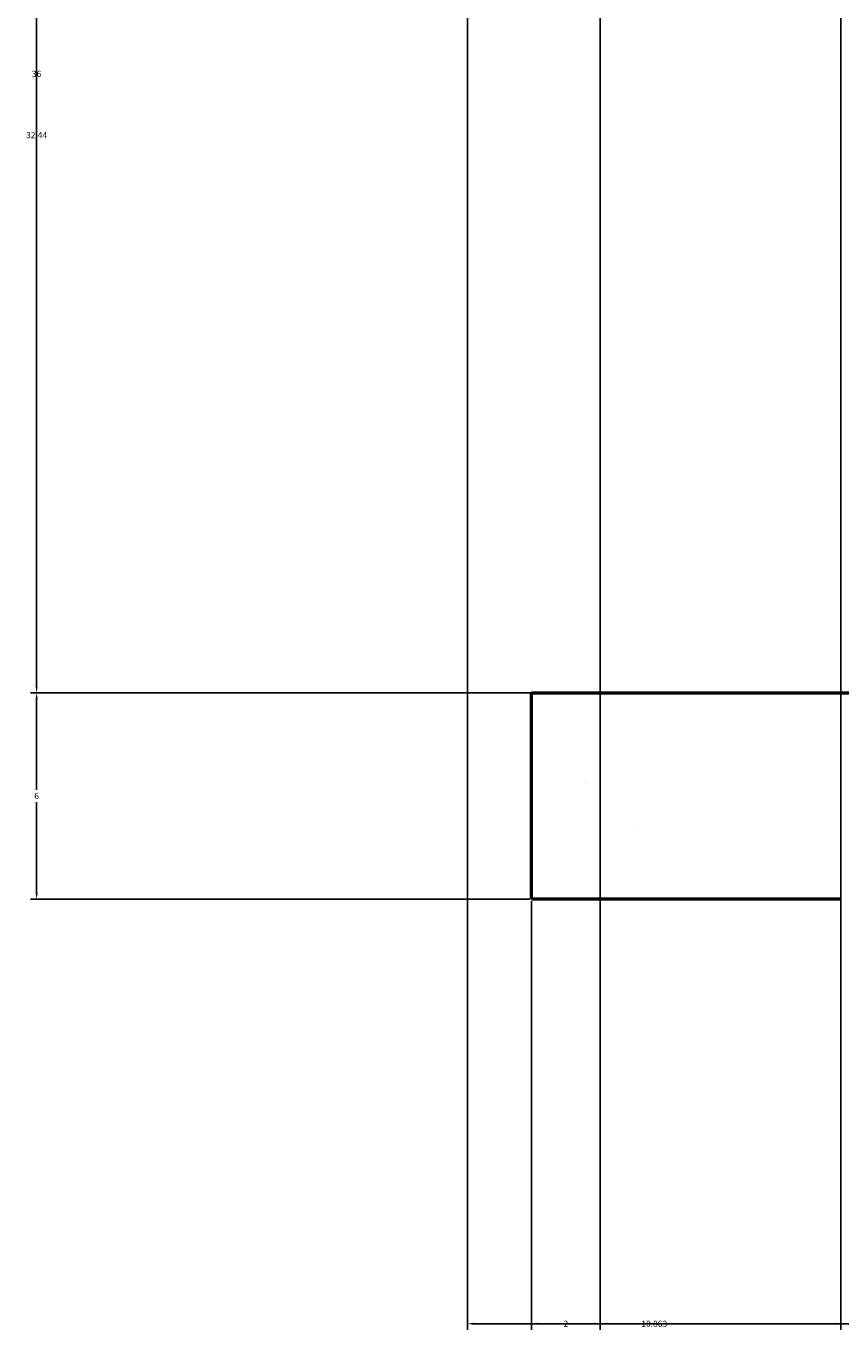
# Model space of a CAD drawing. Units: inches. Extents: x 2812 to 3051, y 1398 to 1659.
# Tile 1 of 65: x 2812 to 2835, y 1398 to 1435. Entities that reach past the tile are written whole.
import ezdxf

# ---------------------------------------------------------------- set-up
doc = ezdxf.new("R2010")
doc.units = ezdxf.units.IN
for name, color, linetype, lineweight in [('A-ANNO-DIMS', 2, 'Continuous', 18), ('S-CONC', 7, 'Continuous', 50), ('S-CONC-PATT', 8, 'Continuous', 18)]:
    doc.layers.add(name, color=color, linetype=linetype, lineweight=lineweight)
doc.styles.get("Standard").update_dxf_attribs({"font": 'arial.ttf'})
doc.dimstyles.get("Standard").update_dxf_attribs({"dimtxt": 0.18, "dimasz": 0.18, "dimexe": 0.18, "dimexo": 0.0625, "dimgap": 0.09, "dimtad": 0, "dimtih": 1, "dimtoh": 1, "dimdec": 4, "dimzin": 0, "dimdsep": 46, "dimtxsty": 'Standard', "dimcen": 0.09, "dimadec": 0, "dimazin": 0, "dimtfac": 1, "dimtdec": 4, "dimtofl": 0, "dimtmove": 0, "dimatfit": 3, "dimfxl": 1, "dimtolj": 1, "dimtzin": 0, "dimarcsym": 0})

# ---------------------------------------------------------------- blocks, each defined once
blk = doc.blocks.new('*D27')
at = {"layer": 'A-ANNO-DIMS', "color": 0, "lineweight": -2, "transparency": 16777216}
for p, q in [((2824.521, 1594.167), (2824.521, 1397.505)), ((2835.385, 1550.757), (2835.385, 1397.505)), ((2824.701, 1397.685), (2829.498, 1397.685)), ((2835.205, 1397.685), (2830.408, 1397.685))]:
    blk.add_line(p, q, dxfattribs=at)
at = {"layer": 'A-ANNO-DIMS', "color": 0, "transparency": 16777216}
for points in [[(2824.701, 1397.715), (2824.701, 1397.655), (2824.521, 1397.685)], [(2835.205, 1397.715), (2835.205, 1397.655), (2835.385, 1397.685)]]:
    blk.add_solid(points, dxfattribs=at)
at = {"layer": 'Defpoints', "color": 0, "transparency": 16777216}
for p in [(2824.521, 1594.23), (2835.385, 1550.82), (2835.385, 1397.685)]:
    blk.add_point(p, dxfattribs=at)
at = {"layer": 'A-ANNO-DIMS', "color": 0, "transparency": 16777216, "insert": (2829.953, 1397.685), "char_height": 0.18, "attachment_point": 5}
blk.add_mtext('\\A1;10.863', dxfattribs=at)
blk = doc.blocks.new('*D41')
at = {"layer": 'A-ANNO-DIMS', "color": 0, "lineweight": -2, "transparency": 16777216}
for p, q in [((2828.385, 1489.973), (2828.385, 1397.505)), ((2826.385, 1409.973), (2826.385, 1397.505)), ((2826.565, 1397.685), (2827.235, 1397.685)), ((2828.205, 1397.685), (2827.535, 1397.685))]:
    blk.add_line(p, q, dxfattribs=at)
at = {"layer": 'A-ANNO-DIMS', "color": 0, "transparency": 16777216}
for points in [[(2826.565, 1397.715), (2826.565, 1397.655), (2826.385, 1397.685)], [(2828.205, 1397.715), (2828.205, 1397.655), (2828.385, 1397.685)]]:
    blk.add_solid(points, dxfattribs=at)
at = {"layer": 'Defpoints', "color": 0, "transparency": 16777216}
for p in [(2828.385, 1490.035), (2826.385, 1410.035), (2828.385, 1397.685)]:
    blk.add_point(p, dxfattribs=at)
at = {"layer": 'A-ANNO-DIMS', "color": 0, "transparency": 16777216, "insert": (2827.385, 1397.685), "char_height": 0.18, "attachment_point": 5}
blk.add_mtext('\\A1;2', dxfattribs=at)
blk = doc.blocks.new('*D42')
at = {"layer": 'A-ANNO-DIMS', "color": 0, "lineweight": -2, "transparency": 16777216}
for p, q in [((2828.385, 1489.973), (2828.385, 1397.505)), ((2847.686, 1487.973), (2847.686, 1397.505)), ((2828.565, 1397.685), (2837.72, 1397.685)), ((2847.506, 1397.685), (2838.351, 1397.685))]:
    blk.add_line(p, q, dxfattribs=at)
at = {"layer": 'A-ANNO-DIMS', "color": 0, "transparency": 16777216}
for points in [[(2828.565, 1397.715), (2828.565, 1397.655), (2828.385, 1397.685)], [(2847.506, 1397.715), (2847.506, 1397.655), (2847.686, 1397.685)]]:
    blk.add_solid(points, dxfattribs=at)
at = {"layer": 'Defpoints', "color": 0, "transparency": 16777216}
for p in [(2828.385, 1490.035), (2847.686, 1488.035), (2847.686, 1397.685)]:
    blk.add_point(p, dxfattribs=at)
at = {"layer": 'A-ANNO-DIMS', "color": 0, "transparency": 16777216, "insert": (2838.036, 1397.685), "char_height": 0.18, "attachment_point": 5}
blk.add_mtext('\\A1;19.3', dxfattribs=at)
blk = doc.blocks.new('*D49')
at = {"layer": 'A-ANNO-DIMS', "color": 0, "lineweight": -2, "transparency": 16777216}
for p, q in [((2826.322, 1416.035), (2811.806, 1416.035)), ((2811.986, 1415.855), (2811.986, 1413.217)), ((2811.986, 1410.215), (2811.986, 1412.853)), ((2826.322, 1410.035), (2811.806, 1410.035))]:
    blk.add_line(p, q, dxfattribs=at)
at = {"layer": 'A-ANNO-DIMS', "color": 0, "transparency": 16777216}
for points in [[(2811.956, 1415.855), (2812.016, 1415.855), (2811.986, 1416.035)], [(2811.956, 1410.215), (2812.016, 1410.215), (2811.986, 1410.035)]]:
    blk.add_solid(points, dxfattribs=at)
at = {"layer": 'Defpoints', "color": 0, "transparency": 16777216}
for p in [(2811.986, 1416.035), (2826.385, 1416.035), (2826.385, 1410.035)]:
    blk.add_point(p, dxfattribs=at)
at = {"layer": 'A-ANNO-DIMS', "color": 0, "transparency": 16777216, "insert": (2811.986, 1413.035), "char_height": 0.18, "attachment_point": 5}
blk.add_mtext('\\A1;6', dxfattribs=at)
blk = doc.blocks.new('*D50')
at = {"layer": 'A-ANNO-DIMS', "color": 0, "lineweight": -2, "transparency": 16777216}
for p, q in [((2835.322, 1462.303), (2811.806, 1462.303)), ((2811.986, 1462.123), (2811.986, 1439.351)), ((2811.986, 1416.215), (2811.986, 1438.987)), ((2835.322, 1416.035), (2811.806, 1416.035))]:
    blk.add_line(p, q, dxfattribs=at)
at = {"layer": 'A-ANNO-DIMS', "color": 0, "transparency": 16777216}
for points in [[(2811.956, 1462.123), (2812.016, 1462.123), (2811.986, 1462.303)], [(2811.956, 1416.215), (2812.016, 1416.215), (2811.986, 1416.035)]]:
    blk.add_solid(points, dxfattribs=at)
at = {"layer": 'Defpoints', "color": 0, "transparency": 16777216}
for p in [(2811.986, 1462.303), (2835.385, 1462.303), (2835.385, 1416.035)]:
    blk.add_point(p, dxfattribs=at)
at = {"layer": 'A-ANNO-DIMS', "color": 0, "transparency": 16777216, "insert": (2811.986, 1439.169), "char_height": 0.18, "attachment_point": 5}
blk.add_mtext('\\A1;46.27', dxfattribs=at)
blk = doc.blocks.new('*D56')
at = {"layer": 'A-ANNO-DIMS', "color": 0, "lineweight": -2, "transparency": 16777216}
for p, q in [((2880.322, 1452.035), (2811.806, 1452.035)), ((2811.986, 1451.855), (2811.986, 1434.217)), ((2811.986, 1416.215), (2811.986, 1433.853)), ((2952.322, 1416.035), (2811.806, 1416.035))]:
    blk.add_line(p, q, dxfattribs=at)
at = {"layer": 'A-ANNO-DIMS', "color": 0, "transparency": 16777216}
for points in [[(2811.956, 1451.855), (2812.016, 1451.855), (2811.986, 1452.035)], [(2811.956, 1416.215), (2812.016, 1416.215), (2811.986, 1416.035)]]:
    blk.add_solid(points, dxfattribs=at)
at = {"layer": 'Defpoints', "color": 0, "transparency": 16777216}
for p in [(2811.986, 1452.035), (2880.385, 1452.035), (2952.385, 1416.035)]:
    blk.add_point(p, dxfattribs=at)
at = {"layer": 'A-ANNO-DIMS', "color": 0, "transparency": 16777216, "insert": (2811.986, 1434.035), "char_height": 0.18, "attachment_point": 5}
blk.add_mtext('\\A1;36', dxfattribs=at)
blk = doc.blocks.new('*D75')
at = {"layer": 'A-ANNO-DIMS', "color": 0, "lineweight": -2, "transparency": 16777216}
for p, q in [((2963.812, 1448.474), (2811.806, 1448.474)), ((2811.986, 1448.294), (2811.986, 1432.437)), ((2811.986, 1416.215), (2811.986, 1432.073)), ((2961.322, 1416.035), (2811.806, 1416.035))]:
    blk.add_line(p, q, dxfattribs=at)
at = {"layer": 'A-ANNO-DIMS', "color": 0, "transparency": 16777216}
for points in [[(2811.956, 1448.294), (2812.016, 1448.294), (2811.986, 1448.474)], [(2811.956, 1416.215), (2812.016, 1416.215), (2811.986, 1416.035)]]:
    blk.add_solid(points, dxfattribs=at)
at = {"layer": 'Defpoints', "color": 0, "transparency": 16777216}
for p in [(2811.986, 1448.474), (2963.874, 1448.474), (2961.385, 1416.035)]:
    blk.add_point(p, dxfattribs=at)
at = {"layer": 'A-ANNO-DIMS', "color": 0, "transparency": 16777216, "insert": (2811.986, 1432.255), "char_height": 0.18, "attachment_point": 5}
blk.add_mtext('\\A1;32.44', dxfattribs=at)

msp = doc.modelspace()

# ---------------------------------------------------------------- hatches: boundary and pattern name
at = {"layer": 'S-CONC-PATT'}
h = msp.add_hatch(dxfattribs=at)
h.set_pattern_fill('AR-SAND', color=256, scale=0.3)
h.paths.add_polyline_path([(3036.3849, 1416.0354), (3027.3849, 1416.0354), (2826.3849, 1416.0354), (2826.3849, 1410.0354), (2835.3849, 1410.0354), (3036.3849, 1410.0354)])
h.paths.add_polyline_path([(2970.3849, 1488.0354), (2969.3849, 1488.0354), (2941.3849, 1488.0354), (2941.3849, 1482.0354), (2970.3849, 1482.0354)])
h.paths.add_polyline_path([(3036.3849, 1488.0354), (3035.3849, 1488.0354), (3006.3849, 1488.0354), (3006.3849, 1482.0354), (3027.3849, 1482.0354), (3036.3849, 1482.0354)])
h.paths.add_polyline_path([(3034.3849, 1490.0354), (3008.3849, 1490.0354), (3008.3849, 1489.0354), (3034.3849, 1489.0354)])
h.paths.add_polyline_path([(3035.3849, 1489.0354), (3034.3849, 1489.0354), (3007.3849, 1489.0354), (3007.3849, 1488.0354), (3035.3849, 1488.0354)])
h.paths.add_polyline_path([(2968.3849, 1490.0354), (2943.3849, 1490.0354), (2943.3849, 1489.0354), (2968.3849, 1489.0354)])
h.paths.add_polyline_path([(2969.3849, 1489.0354), (2968.3849, 1489.0354), (2942.3849, 1489.0354), (2942.3849, 1488.0354), (2969.3849, 1488.0354)])
h.paths.add_polyline_path([(2896.3849, 1488.0354), (2826.3849, 1488.0354), (2826.3849, 1482.0354), (2896.3849, 1482.0354)])
h.paths.add_polyline_path([(2895.3849, 1489.0354), (2894.3849, 1489.0354), (2827.3849, 1489.0354), (2827.3849, 1488.0354), (2895.3849, 1488.0354)])
h.paths.add_polyline_path([(2894.3849, 1490.0354), (2828.3849, 1490.0354), (2828.3849, 1489.0354), (2894.3849, 1489.0354)])
h = msp.add_hatch(dxfattribs=at)
h.set_pattern_fill('AR-CONC', color=256, scale=0.3)
h.paths.add_polyline_path([(3036.3849, 1416.0354), (3027.3849, 1416.0354), (2826.3849, 1416.0354), (2826.3849, 1410.0354), (2835.3849, 1410.0354), (3036.3849, 1410.0354)])

# ---------------------------------------------------------------- linework, layer by layer
at = {"layer": 'S-CONC'}
for p, q in [((2826.3849, 1410.0354), (2826.3849, 1416.0354)), ((2826.3849, 1416.0354), (3027.3849, 1416.0354)), ((2835.3849, 1410.0354), (2826.3849, 1410.0354))]:
    msp.add_line(p, q, dxfattribs=at)

# ---------------------------------------------------------------- dimensions: what is measured, and where the dimension line sits
at = {"layer": 'A-ANNO-DIMS'}
for base, p1, p2, override, picture, middle in [((2835.384907, 1397.685398), (2824.521409, 1594.229631), (2835.384907, 1550.819971), {"dimdec": 3, "dimlfac": 1, "dimrnd": 0, "dimzin": 0, "dimdsep": 46, "dimlunit": 2}, '*D27', (2829.953158, 1397.685398)), ((2828.3849, 1397.6854), (2826.3849, 1410.0354), (2828.3849, 1490.0354), {"dimdec": 0, "dimlfac": 1, "dimrnd": 0, "dimzin": 0, "dimdsep": 46, "dimlunit": 2}, '*D41', (2827.3849, 1397.6854)), ((2847.6863, 1397.6854), (2828.3849, 1490.0354), (2847.6863, 1488.0354), {"dimdec": 1, "dimlfac": 1, "dimrnd": 0, "dimzin": 0, "dimdsep": 46, "dimlunit": 2}, '*D42', (2838.0356, 1397.6854))]:
    dim = msp.add_linear_dim(base=base, p1=p1, p2=p2, dimstyle='Standard', override=override, dxfattribs=at)
    dim.commit()
    dim.dimension.update_dxf_attribs({"geometry": picture, "text_midpoint": middle})
for base, p1, p2, override, picture, middle in [((2811.9855, 1462.3026), (2835.3849, 1416.0354), (2835.3849, 1462.3026), {"dimdec": 2, "dimlfac": 1, "dimrnd": 0, "dimzin": 0, "dimdsep": 46, "dimlunit": 2}, '*D50', (2811.9855, 1439.169)), ((2811.9855, 1452.0354), (2952.3849, 1416.0354), (2880.3849, 1452.0354), {"dimdec": 0, "dimlfac": 1, "dimrnd": 0, "dimzin": 0, "dimdsep": 46, "dimlunit": 2}, '*D56', (2811.9855, 1434.0354)), ((2811.9855, 1448.4738), (2961.3849, 1416.0354), (2963.8741, 1448.4738), {"dimdec": 2, "dimlfac": 1, "dimrnd": 0, "dimzin": 0, "dimdsep": 46, "dimlunit": 2}, '*D75', (2811.9855, 1432.2546)), ((2811.9855, 1416.0354), (2826.3849, 1410.0354), (2826.3849, 1416.0354), {"dimdec": 0, "dimlfac": 1, "dimrnd": 0, "dimzin": 0, "dimdsep": 46, "dimlunit": 2}, '*D49', (2811.9855, 1413.0354))]:
    dim = msp.add_linear_dim(base=base, p1=p1, p2=p2, angle=90, dimstyle='Standard', override=override, dxfattribs=at)
    dim.commit()
    dim.dimension.update_dxf_attribs({"geometry": picture, "text_midpoint": middle})

doc.saveas('drawing.dxf')
